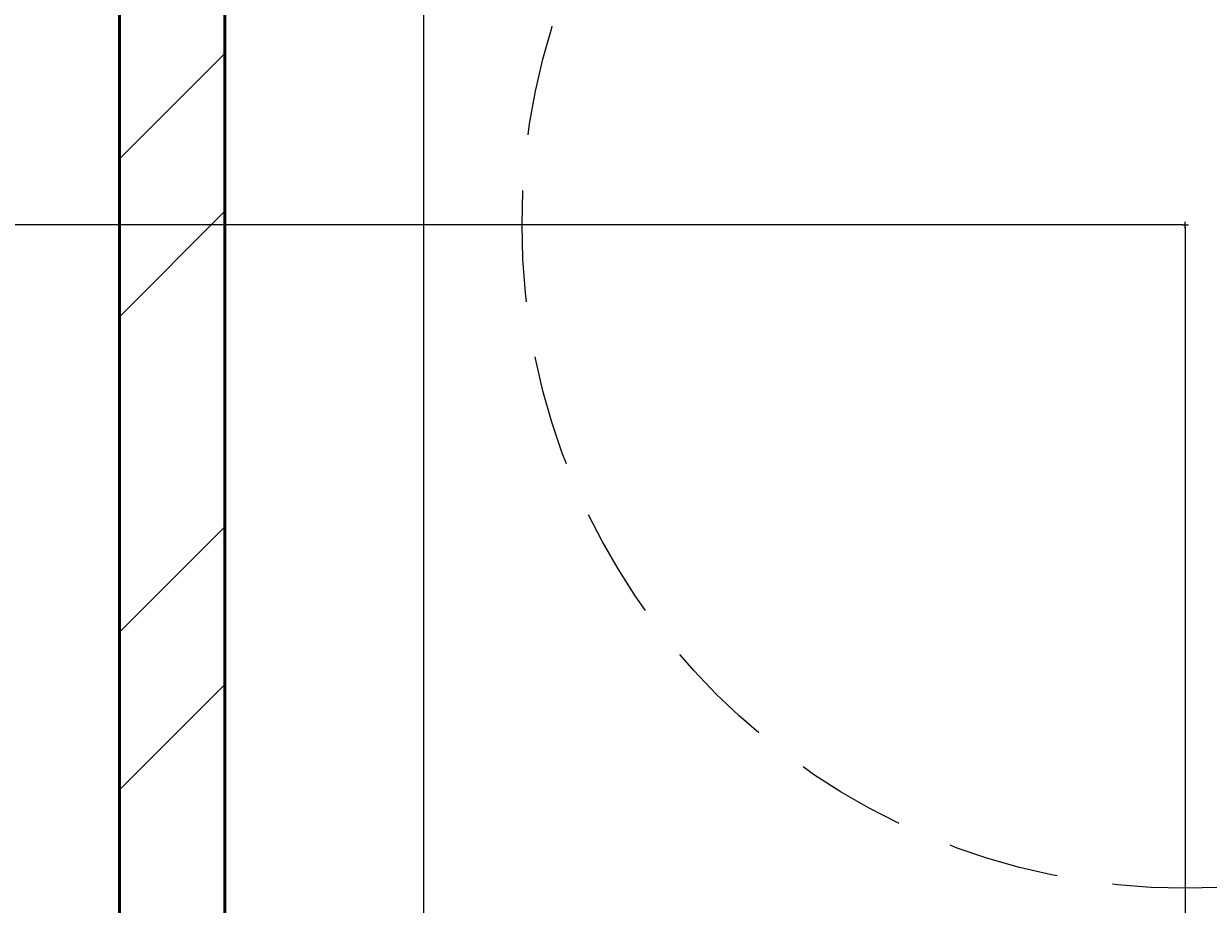
# Model space of a CAD drawing. Units: inches. Extents: x 2812 to 3051, y 1398 to 1659.
# Tile 51 of 65: x 2878 to 2911, y 1579 to 1605. Entities that reach past the tile are written whole.
import ezdxf

# ---------------------------------------------------------------- set-up
doc = ezdxf.new("R2010")
doc.units = ezdxf.units.IN
doc.linetypes.add('HIDDEN2', pattern=[4.7625, 3.175, -1.5875])
for name, color, linetype, lineweight in [('A-ANNO-DIMS', 2, 'Continuous', 18), ('S-CONC', 7, 'Continuous', 50), ('S-CONC-HIDN', 8, 'HIDDEN2', 25), ('S-CONC-PATT', 8, 'Continuous', 18)]:
    doc.layers.add(name, color=color, linetype=linetype, lineweight=lineweight)
doc.styles.get("Standard").update_dxf_attribs({"font": 'arial.ttf'})
doc.dimstyles.get("Standard").update_dxf_attribs({"dimtxt": 0.18, "dimasz": 0.18, "dimexe": 0.18, "dimexo": 0.0625, "dimgap": 0.09, "dimtad": 0, "dimtih": 1, "dimtoh": 1, "dimdec": 4, "dimzin": 0, "dimdsep": 46, "dimtxsty": 'Standard', "dimcen": 0.09, "dimadec": 0, "dimazin": 0, "dimtfac": 1, "dimtdec": 4, "dimtofl": 0, "dimtmove": 0, "dimatfit": 3, "dimfxl": 1, "dimtolj": 1, "dimtzin": 0, "dimarcsym": 0})

# ---------------------------------------------------------------- blocks, each defined once
blk = doc.blocks.new('*D29')
at = {"layer": 'A-ANNO-DIMS', "color": 0, "lineweight": -2, "transparency": 16777216}
for p, q in [((2910.742, 1598.757), (2910.742, 1397.505)), ((2883.385, 1559.757), (2883.385, 1397.505)), ((2883.565, 1397.685), (2896.598, 1397.685)), ((2910.562, 1397.685), (2897.528, 1397.685))]:
    blk.add_line(p, q, dxfattribs=at)
at = {"layer": 'A-ANNO-DIMS', "color": 0, "transparency": 16777216}
for points in [[(2883.565, 1397.715), (2883.565, 1397.655), (2883.385, 1397.685)], [(2910.562, 1397.715), (2910.562, 1397.655), (2910.742, 1397.685)]]:
    blk.add_solid(points, dxfattribs=at)
at = {"layer": 'Defpoints', "color": 0, "transparency": 16777216}
for p in [(2910.742, 1598.82), (2883.385, 1559.82), (2910.742, 1397.685)]:
    blk.add_point(p, dxfattribs=at)
at = {"layer": 'A-ANNO-DIMS', "color": 0, "transparency": 16777216, "insert": (2897.063, 1397.685), "char_height": 0.18, "attachment_point": 5}
blk.add_mtext('\\A1;27.357', dxfattribs=at)
blk = doc.blocks.new('*D37')
at = {"layer": 'A-ANNO-DIMS', "color": 0, "lineweight": -2, "transparency": 16777216}
for p, q in [((2910.679, 1598.82), (2811.806, 1598.82)), ((2811.986, 1598.64), (2811.986, 1579.502)), ((2811.986, 1560), (2811.986, 1579.138)), ((2883.322, 1559.82), (2811.806, 1559.82))]:
    blk.add_line(p, q, dxfattribs=at)
at = {"layer": 'A-ANNO-DIMS', "color": 0, "transparency": 16777216}
for points in [[(2811.956, 1598.64), (2812.016, 1598.64), (2811.986, 1598.82)], [(2811.956, 1560), (2812.016, 1560), (2811.986, 1559.82)]]:
    blk.add_solid(points, dxfattribs=at)
at = {"layer": 'Defpoints', "color": 0, "transparency": 16777216}
for p in [(2811.986, 1598.82), (2910.742, 1598.82), (2883.385, 1559.82)]:
    blk.add_point(p, dxfattribs=at)
at = {"layer": 'A-ANNO-DIMS', "color": 0, "transparency": 16777216, "insert": (2811.986, 1579.32), "char_height": 0.18, "attachment_point": 5}
blk.add_mtext('\\A1;39', dxfattribs=at)
blk = doc.blocks.new('*D38')
at = {"layer": 'A-ANNO-DIMS', "color": 0, "lineweight": -2, "transparency": 16777216}
for p, q in [((2896.322, 1625.82), (2811.806, 1625.82)), ((2811.986, 1625.64), (2811.986, 1612.5)), ((2811.986, 1599), (2811.986, 1612.14)), ((2910.679, 1598.82), (2811.806, 1598.82))]:
    blk.add_line(p, q, dxfattribs=at)
at = {"layer": 'A-ANNO-DIMS', "color": 0, "transparency": 16777216}
for points in [[(2811.956, 1625.64), (2812.016, 1625.64), (2811.986, 1625.82)], [(2811.956, 1599), (2812.016, 1599), (2811.986, 1598.82)]]:
    blk.add_solid(points, dxfattribs=at)
at = {"layer": 'Defpoints', "color": 0, "transparency": 16777216}
for p in [(2811.986, 1625.82), (2896.385, 1625.82), (2910.742, 1598.82)]:
    blk.add_point(p, dxfattribs=at)
at = {"layer": 'A-ANNO-DIMS', "color": 0, "transparency": 16777216, "insert": (2811.986, 1612.32), "char_height": 0.18, "attachment_point": 5}
blk.add_mtext('\\A1;27', dxfattribs=at)
blk = doc.blocks.new('*D58')
at = {"layer": 'A-ANNO-DIMS', "color": 0, "lineweight": -2, "transparency": 16777216}
for p, q in [((2880.385, 1472.098), (2880.385, 1659.35)), ((2883.385, 1472.098), (2883.385, 1659.35)), ((2880.565, 1659.17), (2881.736, 1659.17)), ((2883.205, 1659.17), (2882.034, 1659.17))]:
    blk.add_line(p, q, dxfattribs=at)
at = {"layer": 'A-ANNO-DIMS', "color": 0, "transparency": 16777216}
for points in [[(2880.565, 1659.2), (2880.565, 1659.14), (2880.385, 1659.17)], [(2883.205, 1659.2), (2883.205, 1659.14), (2883.385, 1659.17)]]:
    blk.add_solid(points, dxfattribs=at)
at = {"layer": 'Defpoints', "color": 0, "transparency": 16777216}
for p in [(2883.385, 1659.17), (2880.385, 1472.035), (2883.385, 1472.035)]:
    blk.add_point(p, dxfattribs=at)
at = {"layer": 'A-ANNO-DIMS', "color": 0, "transparency": 16777216, "insert": (2881.885, 1659.17), "char_height": 0.18, "attachment_point": 5}
blk.add_mtext('\\A1;3', dxfattribs=at)
blk = doc.blocks.new('*D59')
at = {"layer": 'A-ANNO-DIMS', "color": 0, "lineweight": -2, "transparency": 16777216}
for p, q in [((2883.385, 1452.098), (2883.385, 1659.35)), ((2889.058, 1467.465), (2889.058, 1659.35)), ((2883.565, 1659.17), (2885.828, 1659.17)), ((2888.878, 1659.17), (2886.615, 1659.17))]:
    blk.add_line(p, q, dxfattribs=at)
at = {"layer": 'A-ANNO-DIMS', "color": 0, "transparency": 16777216}
for points in [[(2883.565, 1659.2), (2883.565, 1659.14), (2883.385, 1659.17)], [(2888.878, 1659.2), (2888.878, 1659.14), (2889.058, 1659.17)]]:
    blk.add_solid(points, dxfattribs=at)
at = {"layer": 'Defpoints', "color": 0, "transparency": 16777216}
for p in [(2889.058, 1659.17), (2889.058, 1467.402), (2883.385, 1452.035)]:
    blk.add_point(p, dxfattribs=at)
at = {"layer": 'A-ANNO-DIMS', "color": 0, "transparency": 16777216, "insert": (2886.221, 1659.17), "char_height": 0.18, "attachment_point": 5}
blk.add_mtext('\\A1;5.673', dxfattribs=at)
blk = doc.blocks.new('*D84')
at = {"layer": 'A-ANNO-DIMS', "color": 0, "lineweight": -2, "transparency": 16777216}
for p, q in [((2910.652, 1598.82), (2910.832, 1598.82)), ((2910.742, 1598.73), (2910.742, 1598.91)), ((2940.963, 1598.82), (2929.81, 1598.82))]:
    blk.add_line(p, q, dxfattribs=at)
at = {"layer": 'A-ANNO-DIMS', "color": 0, "transparency": 16777216}
blk.add_solid([(2929.81, 1598.85), (2929.81, 1598.79), (2929.63, 1598.82)], dxfattribs=at)
at = {"layer": 'Defpoints', "color": 0, "transparency": 16777216}
for p in [(2891.853, 1598.82), (2929.63, 1598.82)]:
    blk.add_point(p, dxfattribs=at)
at = {"layer": 'A-ANNO-DIMS', "color": 0, "transparency": 16777216, "insert": (2941.455, 1598.82), "char_height": 0.18, "attachment_point": 5}
blk.add_mtext('\\A1;∅37.78', dxfattribs=at)

msp = doc.modelspace()

# ---------------------------------------------------------------- hatches: boundary and pattern name
at = {"layer": 'S-CONC-PATT'}
h = msp.add_hatch(dxfattribs=at)
h.set_pattern_fill('ANSI32', color=256)
h.paths.add_polyline_path([(2961.3849, 1637.82), (2952.3849, 1637.82), (2952.3849, 1603.2541), (2961.3849, 1603.2541)])
h.paths.add_polyline_path([(2961.3849, 1594.2541), (2952.3849, 1594.2541), (2952.3849, 1559.82), (2961.3849, 1559.82)])
h.paths.add_polyline_path([(2883.3849, 1637.82), (2880.3849, 1637.82), (2880.3849, 1559.82), (2883.3849, 1559.82)])

# ---------------------------------------------------------------- linework, layer by layer
at = {"layer": 'S-CONC'}
for p, q in [((2880.3849, 1637.82), (2880.3849, 1559.82)), ((2883.3849, 1637.82), (2883.3849, 1559.82))]:
    msp.add_line(p, q, dxfattribs=at)
at = {"layer": 'S-CONC-HIDN'}
msp.add_circle((2910.7415, 1598.82), 18.8884, dxfattribs=at)

# ---------------------------------------------------------------- dimensions: what is measured, and where the dimension line sits
at = {"layer": 'A-ANNO-DIMS'}
for base, p1, p2, override, picture, middle in [((2883.3849, 1659.17), (2880.3849, 1472.0354), (2883.3849, 1472.0354), {"dimdec": 0, "dimlfac": 1, "dimrnd": 0, "dimzin": 0, "dimdsep": 46, "dimlunit": 2}, '*D58', (2881.8849, 1659.17)), ((2889.0577, 1659.17), (2883.3849, 1452.0354), (2889.0577, 1467.4024), {"dimdec": 3, "dimlfac": 1, "dimrnd": 0, "dimzin": 0, "dimdsep": 46, "dimlunit": 2}, '*D59', (2886.2213, 1659.17)), ((2910.7415, 1397.6854), (2883.3849, 1559.82), (2910.7415, 1598.82), {"dimdec": 3, "dimlfac": 1, "dimrnd": 0, "dimzin": 0, "dimdsep": 46, "dimlunit": 2}, '*D29', (2897.0632, 1397.6854))]:
    dim = msp.add_linear_dim(base=base, p1=p1, p2=p2, dimstyle='Standard', override=override, dxfattribs=at)
    dim.commit()
    dim.dimension.update_dxf_attribs({"geometry": picture, "text_midpoint": middle})
for base, p1, p2, picture, middle in [((2811.9855, 1625.82), (2910.7415, 1598.82), (2896.3849, 1625.82), '*D38', (2811.9855, 1612.32)), ((2811.9855, 1598.82), (2883.3849, 1559.82), (2910.7415, 1598.82), '*D37', (2811.9855, 1579.32))]:
    dim = msp.add_linear_dim(base=base, p1=p1, p2=p2, angle=90, dimstyle='Standard', override={"dimdec": 0, "dimlfac": 1, "dimrnd": 0, "dimzin": 0, "dimdsep": 46, "dimlunit": 2}, dxfattribs=at)
    dim.commit()
    dim.dimension.update_dxf_attribs({"geometry": picture, "text_midpoint": middle})
dim = msp.add_diameter_dim_2p(p1=(2891.8531, 1598.8199), p2=(2929.6299, 1598.82), dimstyle='Standard', override={"dimdec": 2, "dimlfac": 1, "dimrnd": 0, "dimzin": 0, "dimdsep": 46, "dimlunit": 2}, dxfattribs=at)
dim.commit()
dim.dimension.update_dxf_attribs({"geometry": '*D84', "text_midpoint": (2940.963, 1598.82), "dimtype": 163})

doc.saveas('drawing.dxf')
